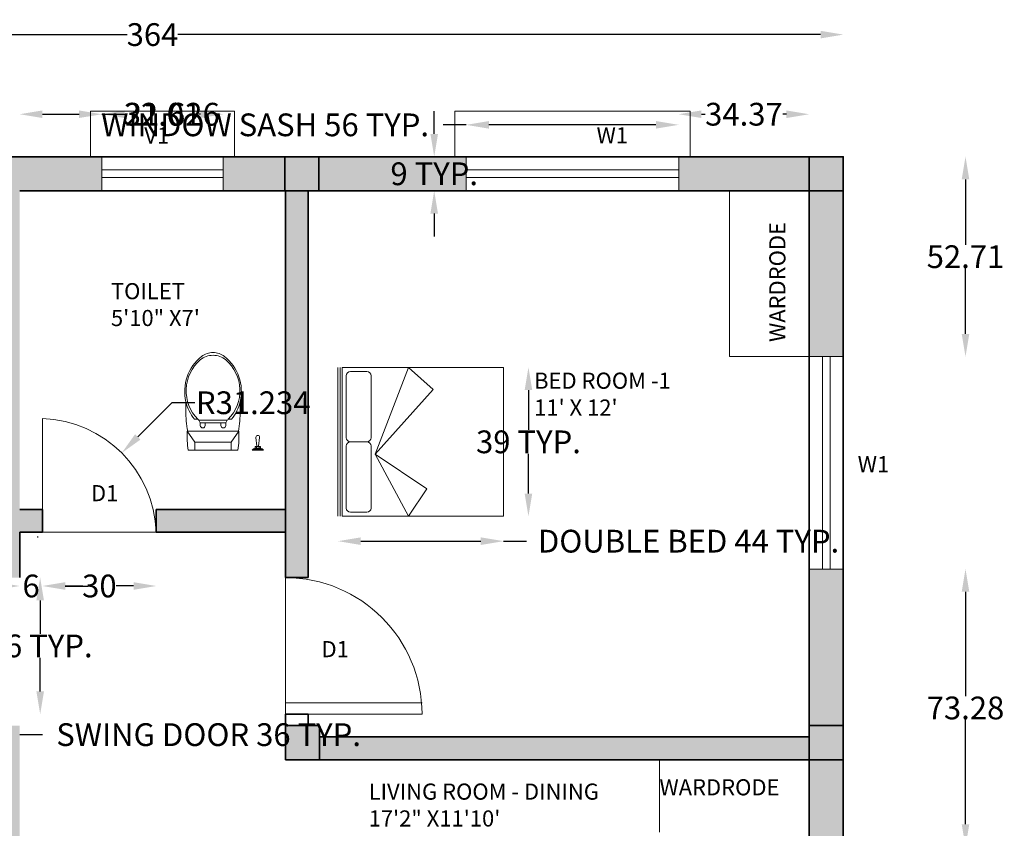
# Model space of a CAD drawing. Units: inches. Extents: x 1994 to 3075, y 3517 to 3950.
# Tile 58 of 58: x 2816 to 3075, y 3737 to 3950. Entities that reach past the tile are written whole.
import ezdxf

# ---------------------------------------------------------------- set-up
doc = ezdxf.new("R2010")
doc.units = ezdxf.units.IN
for name, color, linetype, lineweight in [('A-ANNO-DIMS', 2, 'Continuous', 18), ('A-ANNO-TEXT', 7, 'Continuous', 18), ('A-AREA-IDEN', 7, 'Continuous', 18), ('A-COLS', 7, 'Continuous', 35), ('A-COLS-PATT', 6, 'Continuous', 13), ('A-DOOR', 3, 'Continuous', 18), ('A-FLOR-CASE', 8, 'Continuous', 18), ('A-FURN', 8, 'Continuous', 18), ('A-GLAZ', 4, 'Continuous', 18), ('A-GLAZ-PROJ', 4, 'Continuous', 18), ('A-WALL', 7, 'Continuous', 35), ('A-WALL-PATT', 252, 'Continuous', 13), ('WC-Detail_dwgmodels.com', 8, 'Continuous', 13), ('WC-Outline_dwgmodels.com', 8, 'Continuous', 18)]:
    doc.layers.add(name, color=color, linetype=linetype, lineweight=lineweight)
doc.styles.get("Standard").update_dxf_attribs({"font": 'arial.ttf'})
doc.dimstyles.get("Standard").update_dxf_attribs({"dimtxt": 6, "dimasz": 6, "dimexe": 0.18, "dimexo": 0.0625, "dimgap": 0.09, "dimtad": 0, "dimtih": 1, "dimtoh": 1, "dimdec": 4, "dimzin": 0, "dimdsep": 46, "dimlunit": 4, "dimtxsty": 'Standard', "dimcen": 0.09, "dimse1": 1, "dimse2": 1, "dimadec": 0, "dimazin": 0, "dimtfac": 1, "dimtdec": 4, "dimtofl": 0, "dimtmove": 0, "dimatfit": 3, "dimfxl": 1, "dimtolj": 1, "dimtzin": 0, "dimarcsym": 0})

# ---------------------------------------------------------------- blocks, each defined once
blk = doc.blocks.new('DOOR-SWING-36IN')
for p, q in [((36, 0), (36, 36)), ((36, 36), (36, 0)), ((0, 3), (36, 3)), ((36, 0), (0, 0)), ((0, 0), (36, 0))]:
    blk.add_line(p, q)
blk.add_arc((36, 0), 36, 90, 180)
blk = doc.blocks.new('BED-DOUBLE-PLAN')
for p, q in [((0, 39.28), (0, 0)), ((0.55, 0), (0.55, 39.28)), ((1.09, 0), (1.09, 39.28)), ((1.09, 39.28), (43.64, 39.28)), ((9.82, 16.37), (18.55, 39.28)), ((25.06, 33.47), (18.55, 39.28)), ((43.64, 39.28), (43.64, 0)), ((2.18, 20.73), (2.18, 37.09)), ((3.27, 38.19), (7.64, 38.19)), ((8.73, 20.73), (8.73, 37.09)), ((9.82, 16.37), (25.06, 33.47)), ((2.18, 2.18), (2.18, 18.55)), ((7.64, 19.64), (3.27, 19.64)), ((8.73, 2.18), (8.73, 18.55)), ((18.55, 0), (9.82, 16.37)), ((23.41, 7.25), (9.82, 16.37)), ((18.55, 0), (23.41, 7.25)), ((7.64, 1.09), (3.27, 1.09)), ((43.64, 0), (1.09, 0))]:
    blk.add_line(p, q)
for centre, start, end in [((3.27, 37.09), 90, 180), ((7.64, 37.09), 0, 90), ((3.27, 20.73), 180, 270), ((3.27, 18.55), 90, 180), ((7.64, 20.73), 270, 0), ((7.64, 18.55), 0, 90), ((3.27, 2.18), 180, 270), ((7.64, 2.18), 270, 0)]:
    blk.add_arc(centre, 1.09, start, end)
blk = doc.blocks.new('WINDOW-56IN-SASH')
for p, q in [((56.01, 9), (0, 9)), ((0, 5.5), (56.01, 5.5)), ((0, 3.5), (56.01, 3.5)), ((0, 0), (56.01, 0))]:
    blk.add_line(p, q)
blk = doc.blocks.new('WINDOW-HOOD-62IN')
for p, q in [((0, 59.01), (0, 62.01)), ((0, 62.01), (12, 62.01)), ((0, 0), (0, 59.01)), ((12, 0), (0, 0))]:
    blk.add_line(p, q)
blk = doc.blocks.new('*D17')
at = {"layer": 'A-ANNO-DIMS', "color": 0, "lineweight": -2, "transparency": 16777216}
for p, q in [((2933.69, 3922.53), (2927.69, 3922.53)), ((2983.7, 3922.53), (2939.69, 3922.53))]:
    blk.add_line(p, q, dxfattribs=at)
at = {"layer": 'A-ANNO-DIMS', "color": 0, "transparency": 16777216}
for points in [[(2939.69, 3923.53), (2939.69, 3921.53), (2933.69, 3922.53)], [(2983.7, 3923.53), (2983.7, 3921.53), (2989.7, 3922.53)]]:
    blk.add_solid(points, dxfattribs=at)
at = {"layer": 'Defpoints', "color": 0, "transparency": 16777216}
for p in [(2933.69, 3922.53), (2933.69, 3914.13), (2989.7, 3914.13)]:
    blk.add_point(p, dxfattribs=at)
at = {"layer": 'A-ANNO-DIMS', "color": 0, "transparency": 16777216, "insert": (2880.74, 3922.53), "char_height": 6, "attachment_point": 5}
blk.add_mtext('\\A1;WINDOW SASH 56 TYP.', dxfattribs=at)
blk = doc.blocks.new('*D18')
at = {"layer": 'A-ANNO-DIMS', "color": 0, "lineweight": -2, "transparency": 16777216}
for p, q in [((2925.29, 3920.13), (2925.29, 3926.13)), ((2925.29, 3899.13), (2925.29, 3893.13))]:
    blk.add_line(p, q, dxfattribs=at)
at = {"layer": 'A-ANNO-DIMS', "color": 0, "transparency": 16777216}
for points in [[(2924.29, 3920.13), (2926.29, 3920.13), (2925.29, 3914.13)], [(2924.29, 3899.13), (2926.29, 3899.13), (2925.29, 3905.13)]]:
    blk.add_solid(points, dxfattribs=at)
at = {"layer": 'Defpoints', "color": 0, "transparency": 16777216}
for p in [(2933.69, 3914.13), (2925.29, 3905.13), (2933.69, 3905.13)]:
    blk.add_point(p, dxfattribs=at)
at = {"layer": 'A-ANNO-DIMS', "color": 0, "transparency": 16777216, "insert": (2925.29, 3909.63), "char_height": 6, "attachment_point": 5}
blk.add_mtext('\\A1;9 TYP.', dxfattribs=at)
blk = doc.blocks.new('*D21')
at = {"layer": 'A-ANNO-DIMS', "color": 0, "lineweight": -2, "transparency": 16777216}
for p, q in [((2786.07, 3761.73), (2810.07, 3761.73)), ((2816.07, 3761.73), (2822.07, 3761.73))]:
    blk.add_line(p, q, dxfattribs=at)
at = {"layer": 'A-ANNO-DIMS', "color": 0, "transparency": 16777216}
for points in [[(2786.07, 3762.73), (2786.07, 3760.73), (2780.07, 3761.73)], [(2810.07, 3762.73), (2810.07, 3760.73), (2816.07, 3761.73)]]:
    blk.add_solid(points, dxfattribs=at)
at = {"layer": 'Defpoints', "color": 0, "transparency": 16777216}
for p in [(2780.07, 3767.13), (2816.07, 3767.13), (2816.07, 3761.73)]:
    blk.add_point(p, dxfattribs=at)
at = {"layer": 'A-ANNO-DIMS', "color": 0, "transparency": 16777216, "insert": (2865.85, 3761.73), "char_height": 6, "attachment_point": 5}
blk.add_mtext('\\A1;SWING DOOR 36 TYP.', dxfattribs=at)
blk = doc.blocks.new('*D22')
at = {"layer": 'A-ANNO-DIMS', "color": 0, "lineweight": -2, "transparency": 16777216}
for p, q in [((2821.47, 3797.13), (2821.47, 3788.28)), ((2821.47, 3773.13), (2821.47, 3781.97))]:
    blk.add_line(p, q, dxfattribs=at)
at = {"layer": 'A-ANNO-DIMS', "color": 0, "transparency": 16777216}
for points in [[(2820.47, 3797.13), (2822.47, 3797.13), (2821.47, 3803.13)], [(2820.47, 3773.13), (2822.47, 3773.13), (2821.47, 3767.13)]]:
    blk.add_solid(points, dxfattribs=at)
at = {"layer": 'Defpoints', "color": 0, "transparency": 16777216}
for p in [(2816.07, 3803.13), (2821.47, 3803.13), (2816.07, 3767.13)]:
    blk.add_point(p, dxfattribs=at)
at = {"layer": 'A-ANNO-DIMS', "color": 0, "transparency": 16777216, "insert": (2821.47, 3785.13), "char_height": 6, "attachment_point": 5}
blk.add_mtext('\\A1;36 TYP.', dxfattribs=at)
blk = doc.blocks.new('*D23')
at = {"layer": 'A-ANNO-DIMS', "color": 0, "lineweight": -2, "transparency": 16777216}
for p, q in [((2905.93, 3812.75), (2937.57, 3812.75)), ((2943.57, 3812.75), (2949.57, 3812.75))]:
    blk.add_line(p, q, dxfattribs=at)
at = {"layer": 'A-ANNO-DIMS', "color": 0, "transparency": 16777216}
for points in [[(2905.93, 3813.75), (2905.93, 3811.75), (2899.93, 3812.75)], [(2937.57, 3813.75), (2937.57, 3811.75), (2943.57, 3812.75)]]:
    blk.add_solid(points, dxfattribs=at)
at = {"layer": 'Defpoints', "color": 0, "transparency": 16777216}
for p in [(2899.93, 3819.3), (2943.57, 3819.3), (2943.57, 3812.75)]:
    blk.add_point(p, dxfattribs=at)
at = {"layer": 'A-ANNO-DIMS', "color": 0, "transparency": 16777216, "insert": (2992.3, 3812.75), "char_height": 6, "attachment_point": 5}
blk.add_mtext('\\A1;DOUBLE BED 44 TYP.', dxfattribs=at)
blk = doc.blocks.new('*D24')
at = {"layer": 'A-ANNO-DIMS', "color": 0, "lineweight": -2, "transparency": 16777216}
for p, q in [((2950.12, 3852.58), (2950.12, 3842.09)), ((2950.12, 3825.3), (2950.12, 3835.78))]:
    blk.add_line(p, q, dxfattribs=at)
at = {"layer": 'A-ANNO-DIMS', "color": 0, "transparency": 16777216}
for points in [[(2949.12, 3852.58), (2951.12, 3852.58), (2950.12, 3858.58)], [(2949.12, 3825.3), (2951.12, 3825.3), (2950.12, 3819.3)]]:
    blk.add_solid(points, dxfattribs=at)
at = {"layer": 'Defpoints', "color": 0, "transparency": 16777216}
for p in [(2943.57, 3858.58), (2950.12, 3858.58), (2943.57, 3819.3)]:
    blk.add_point(p, dxfattribs=at)
at = {"layer": 'A-ANNO-DIMS', "color": 0, "transparency": 16777216, "insert": (2950.12, 3838.94), "char_height": 6, "attachment_point": 5}
blk.add_mtext('\\A1;39 TYP.', dxfattribs=at)
blk = doc.blocks.new('*D31')
at = {"layer": 'A-ANNO-DIMS', "color": 0, "lineweight": -2, "transparency": 16777216}
for p, q in [((2675.07, 3946.33), (2844.37, 3946.33)), ((3027.07, 3946.33), (2857.78, 3946.33))]:
    blk.add_line(p, q, dxfattribs=at)
at = {"layer": 'A-ANNO-DIMS', "color": 0, "transparency": 16777216}
for points in [[(2675.07, 3947.33), (2675.07, 3945.33), (2669.07, 3946.33)], [(3027.07, 3947.33), (3027.07, 3945.33), (3033.07, 3946.33)]]:
    blk.add_solid(points, dxfattribs=at)
at = {"layer": 'Defpoints', "color": 0, "transparency": 16777216}
for p in [(3033.07, 3946.33), (2669.07, 3914.13), (3033.07, 3914.13)]:
    blk.add_point(p, dxfattribs=at)
at = {"layer": 'A-ANNO-DIMS', "color": 0, "transparency": 16777216, "insert": (2851.07, 3946.33), "char_height": 6, "attachment_point": 5}
blk.add_mtext('\\A1;364', dxfattribs=at)
blk = doc.blocks.new('*D38')
at = {"layer": 'A-ANNO-DIMS', "color": 0, "lineweight": -2, "transparency": 16777216}
for p, q in [((3065.27, 3799.41), (3065.27, 3771.92)), ((3065.27, 3738.12), (3065.27, 3765.61))]:
    blk.add_line(p, q, dxfattribs=at)
at = {"layer": 'A-ANNO-DIMS', "color": 0, "transparency": 16777216}
for points in [[(3064.27, 3799.41), (3066.27, 3799.41), (3065.27, 3805.41)], [(3064.27, 3738.12), (3066.27, 3738.12), (3065.27, 3732.12)]]:
    blk.add_solid(points, dxfattribs=at)
at = {"layer": 'Defpoints', "color": 0, "transparency": 16777216}
for p in [(3033.07, 3805.41), (3065.27, 3805.41), (3033.07, 3732.12)]:
    blk.add_point(p, dxfattribs=at)
at = {"layer": 'A-ANNO-DIMS', "color": 0, "transparency": 16777216, "insert": (3065.27, 3768.77), "char_height": 6, "attachment_point": 5}
blk.add_mtext('\\A1;73.28', dxfattribs=at)
blk = doc.blocks.new('*D39')
at = {"layer": 'A-ANNO-DIMS', "color": 0, "lineweight": -2, "transparency": 16777216}
for p, q in [((3065.27, 3908.13), (3065.27, 3890.93)), ((3065.27, 3867.42), (3065.27, 3884.62))]:
    blk.add_line(p, q, dxfattribs=at)
at = {"layer": 'A-ANNO-DIMS', "color": 0, "transparency": 16777216}
for points in [[(3064.27, 3908.13), (3066.27, 3908.13), (3065.27, 3914.13)], [(3064.27, 3867.42), (3066.27, 3867.42), (3065.27, 3861.42)]]:
    blk.add_solid(points, dxfattribs=at)
at = {"layer": 'Defpoints', "color": 0, "transparency": 16777216}
for p in [(3033.07, 3914.13), (3065.27, 3914.13), (3033.07, 3861.42)]:
    blk.add_point(p, dxfattribs=at)
at = {"layer": 'A-ANNO-DIMS', "color": 0, "transparency": 16777216, "insert": (3065.27, 3887.77), "char_height": 6, "attachment_point": 5}
blk.add_mtext('\\A1;52.71', dxfattribs=at)
blk = doc.blocks.new('*D41')
at = {"layer": 'A-ANNO-DIMS', "color": 0, "lineweight": -2, "transparency": 16777216}
for p, q in [((2822.07, 3925.33), (2831.7, 3925.33)), ((2837.7, 3925.33), (2843.7, 3925.33))]:
    blk.add_line(p, q, dxfattribs=at)
at = {"layer": 'A-ANNO-DIMS', "color": 0, "transparency": 16777216}
for points in [[(2822.07, 3926.33), (2822.07, 3924.33), (2816.07, 3925.33)], [(2831.7, 3926.33), (2831.7, 3924.33), (2837.7, 3925.33)]]:
    blk.add_solid(points, dxfattribs=at)
at = {"layer": 'Defpoints', "color": 0, "transparency": 16777216}
for p in [(2837.7, 3925.33), (2816.07, 3905.13), (2837.7, 3905.13)]:
    blk.add_point(p, dxfattribs=at)
at = {"layer": 'A-ANNO-DIMS', "color": 0, "transparency": 16777216, "insert": (2856.29, 3925.33), "char_height": 6, "attachment_point": 5}
blk.add_mtext('\\A1;21.626', dxfattribs=at)
blk = doc.blocks.new('*D42')
at = {"layer": 'A-ANNO-DIMS', "color": 0, "lineweight": -2, "transparency": 16777216}
for p, q in [((2843.7, 3925.33), (2844.07, 3925.33)), ((2863.71, 3925.33), (2863.34, 3925.33))]:
    blk.add_line(p, q, dxfattribs=at)
at = {"layer": 'A-ANNO-DIMS', "color": 0, "transparency": 16777216}
for points in [[(2843.7, 3926.33), (2843.7, 3924.33), (2837.7, 3925.33)], [(2863.71, 3926.33), (2863.71, 3924.33), (2869.71, 3925.33)]]:
    blk.add_solid(points, dxfattribs=at)
at = {"layer": 'Defpoints', "color": 0, "transparency": 16777216}
for p in [(2869.71, 3925.33), (2837.7, 3905.13), (2869.71, 3905.13)]:
    blk.add_point(p, dxfattribs=at)
at = {"layer": 'A-ANNO-DIMS', "color": 0, "transparency": 16777216, "insert": (2853.7, 3925.33), "char_height": 6, "attachment_point": 5}
blk.add_mtext('\\A1;32.01', dxfattribs=at)
blk = doc.blocks.new('*D43')
at = {"layer": 'A-ANNO-DIMS', "color": 0, "lineweight": -2, "transparency": 16777216}
for p, q in [((2995.7, 3925.33), (2996.68, 3925.33)), ((3018.07, 3925.33), (3017.1, 3925.33))]:
    blk.add_line(p, q, dxfattribs=at)
at = {"layer": 'A-ANNO-DIMS', "color": 0, "transparency": 16777216}
for points in [[(2995.7, 3926.33), (2995.7, 3924.33), (2989.7, 3925.33)], [(3018.07, 3926.33), (3018.07, 3924.33), (3024.07, 3925.33)]]:
    blk.add_solid(points, dxfattribs=at)
at = {"layer": 'Defpoints', "color": 0, "transparency": 16777216}
for p in [(3024.07, 3925.33), (2989.7, 3905.13), (3024.07, 3905.13)]:
    blk.add_point(p, dxfattribs=at)
at = {"layer": 'A-ANNO-DIMS', "color": 0, "transparency": 16777216, "insert": (3006.89, 3925.33), "char_height": 6, "attachment_point": 5}
blk.add_mtext('\\A1;34.37', dxfattribs=at)
blk = doc.blocks.new('*D50')
at = {"layer": 'A-ANNO-DIMS', "color": 0, "lineweight": -2, "transparency": 16777216}
for p, q in [((2828.07, 3800.93), (2832.7, 3800.93)), ((2846.07, 3800.93), (2841.45, 3800.93))]:
    blk.add_line(p, q, dxfattribs=at)
at = {"layer": 'A-ANNO-DIMS', "color": 0, "transparency": 16777216}
for points in [[(2828.07, 3801.93), (2828.07, 3799.93), (2822.07, 3800.93)], [(2846.07, 3801.93), (2846.07, 3799.93), (2852.07, 3800.93)]]:
    blk.add_solid(points, dxfattribs=at)
at = {"layer": 'Defpoints', "color": 0, "transparency": 16777216}
for p in [(2822.07, 3821.13), (2852.07, 3821.13), (2822.07, 3800.93)]:
    blk.add_point(p, dxfattribs=at)
at = {"layer": 'A-ANNO-DIMS', "color": 0, "transparency": 16777216, "insert": (2837.07, 3800.93), "char_height": 6, "attachment_point": 5}
blk.add_mtext('\\A1;30', dxfattribs=at)
blk = doc.blocks.new('*D51')
at = {"layer": 'A-ANNO-DIMS', "color": 0, "lineweight": -2, "transparency": 16777216}
for p, q in [((2810.072038, 3800.926884), (2804.072038, 3800.926884)), ((2828.072038, 3800.926884), (2834.072038, 3800.926884))]:
    blk.add_line(p, q, dxfattribs=at)
at = {"layer": 'A-ANNO-DIMS', "color": 0, "transparency": 16777216}
for points in [[(2810.072038, 3801.926884), (2810.072038, 3799.926884), (2816.072038, 3800.926884)], [(2828.072038, 3801.926884), (2828.072038, 3799.926884), (2822.072038, 3800.926884)]]:
    blk.add_solid(points, dxfattribs=at)
at = {"layer": 'Defpoints', "color": 0, "transparency": 16777216}
for p in [(2816.072038, 3821.126884), (2822.072038, 3821.126884), (2816.072038, 3800.926884)]:
    blk.add_point(p, dxfattribs=at)
at = {"layer": 'A-ANNO-DIMS', "color": 0, "transparency": 16777216, "insert": (2819.072038, 3800.926884), "char_height": 6, "attachment_point": 5}
blk.add_mtext('\\A1;6', dxfattribs=at)
blk = doc.blocks.new('*D55')
at = {"layer": 'A-ANNO-DIMS', "color": 0, "lineweight": -2, "transparency": 16777216}
for p, q in [((2856.2, 3849.25), (2847.19, 3840.24)), ((2862.2, 3849.25), (2856.2, 3849.25)), ((2820.77, 3813.92), (2820.95, 3813.92)), ((2820.86, 3813.83), (2820.86, 3814.01))]:
    blk.add_line(p, q, dxfattribs=at)
at = {"layer": 'A-ANNO-DIMS', "color": 0, "transparency": 16777216}
blk.add_solid([(2846.48, 3840.95), (2847.9, 3839.54), (2842.95, 3836)], dxfattribs=at)
at = {"layer": 'Defpoints', "color": 0, "transparency": 16777216}
for p in [(2842.95, 3836), (2820.86, 3813.92)]:
    blk.add_point(p, dxfattribs=at)
at = {"layer": 'A-ANNO-DIMS', "color": 0, "transparency": 16777216, "insert": (2877.6, 3849.25), "char_height": 6, "attachment_point": 5}
blk.add_mtext('\\A1;R31.234', dxfattribs=at)

msp = doc.modelspace()

# ---------------------------------------------------------------- hatches: boundary and pattern name
at = {"layer": 'A-COLS-PATT'}
h = msp.add_hatch(color=256, dxfattribs=at)
h.dxf.hatch_style = 1
h.paths.add_polyline_path([(2678.072, 3914.1269), (2669.072, 3914.1269), (2669.072, 3905.1269), (2678.072, 3905.1269)])
h.paths.add_polyline_path([(2816.072, 3914.1269), (2807.072, 3914.1269), (2807.072, 3905.1269), (2816.072, 3905.1269)])
h.paths.add_polyline_path([(2894.9096, 3914.1269), (2885.9096, 3914.1269), (2885.9096, 3905.1269), (2894.9096, 3905.1269)])
h.paths.add_polyline_path([(3033.072, 3914.1269), (3024.072, 3914.1269), (3024.072, 3905.1269), (3033.072, 3905.1269)])
h.paths.add_polyline_path([(3033.072, 3764.1269), (3024.072, 3764.1269), (3024.072, 3755.1269), (3033.072, 3755.1269)])
h.paths.add_polyline_path([(2895.072, 3764.1269), (2886.072, 3764.1269), (2886.072, 3755.1269), (2895.072, 3755.1269)])
h.paths.add_polyline_path([(2816.072, 3764.1269), (2807.072, 3764.1269), (2807.072, 3755.1269), (2816.072, 3755.1269)])
h.paths.add_polyline_path([(2678.072, 3764.1269), (2669.072, 3764.1269), (2669.072, 3755.1269), (2678.072, 3755.1269)])
h.paths.add_polyline_path([(2678.072, 3664.1269), (2669.072, 3664.1269), (2669.072, 3655.1269), (2678.072, 3655.1269)])
h.paths.add_polyline_path([(2816.072, 3664.1269), (2807.072, 3664.1269), (2807.072, 3655.1269), (2816.072, 3655.1269)])
h.paths.add_polyline_path([(3033.072, 3616.1269), (3024.072, 3616.1269), (3024.072, 3607.1269), (3033.072, 3607.1269)])
h.paths.add_polyline_path([(2894.9096, 3616.1269), (2885.9096, 3616.1269), (2885.9096, 3607.1269), (2894.9096, 3607.1269)])
h.paths.add_polyline_path([(2816.072, 3559.1269), (2807.072, 3559.1269), (2807.072, 3550.1269), (2816.072, 3550.1269)])
h.paths.add_polyline_path([(2678.072, 3559.1269), (2669.072, 3559.1269), (2669.072, 3550.1269), (2678.072, 3550.1269)])
at = {"layer": 'A-WALL-PATT'}
h = msp.add_hatch(color=256, dxfattribs=at)
h.dxf.hatch_style = 1
h.paths.add_polyline_path([(2678.072, 3755.1269), (2669.072, 3755.1269), (2669.072, 3718.5523), (2678.072, 3718.5523)])
h.paths.add_polyline_path([(2807.072, 3761.1269), (2678.072, 3761.1269), (2678.072, 3755.1269), (2807.072, 3755.1269)])
h.paths.add_polyline_path([(2678.072, 3812.7371), (2669.072, 3812.7371), (2669.072, 3809.7371), (2669.072, 3764.1269), (2678.072, 3764.1269)])
h.paths.add_polyline_path([(2678.072, 3905.1269), (2669.072, 3905.1269), (2669.072, 3868.7491), (2678.072, 3868.7491)])
h.paths.add_polyline_path([(2723.826, 3914.1269), (2720.826, 3914.1269), (2678.072, 3914.1269), (2678.072, 3905.1269), (2723.826, 3905.1269)])
h.paths.add_polyline_path([(2807.072, 3914.1269), (2779.838, 3914.1269), (2779.838, 3905.1269), (2807.072, 3905.1269)])
h.paths.add_polyline_path([(2837.6979, 3914.1269), (2834.6979, 3914.1269), (2820.9062, 3914.1269), (2816.072, 3914.1269), (2816.072, 3905.1269), (2837.6979, 3905.1269)])
h.paths.add_polyline_path([(2885.9096, 3914.1269), (2869.71, 3914.1269), (2869.71, 3905.1269), (2876.9183, 3905.1269), (2885.9096, 3905.1269)])
h.paths.add_polyline_path([(2933.6904, 3914.1269), (2930.6904, 3914.1269), (2894.9096, 3914.1269), (2894.9096, 3905.1269), (2933.6904, 3905.1269)])
h.paths.add_polyline_path([(3024.072, 3914.1269), (2989.7025, 3914.1269), (2989.7025, 3905.1269), (3024.072, 3905.1269)])
h.paths.add_polyline_path([(3033.072, 3905.1269), (3024.072, 3905.1269), (3024.072, 3861.4192), (3033.072, 3861.4192)])
h.paths.add_polyline_path([(3033.072, 3805.4072), (3024.072, 3805.4072), (3024.072, 3764.1269), (3033.072, 3764.1269)])
h.paths.add_polyline_path([(3033.072, 3755.1269), (3024.072, 3755.1269), (3024.072, 3732.1247), (3033.072, 3732.1247), (3033.072, 3735.1247)])
h.paths.add_polyline_path([(3024.072, 3761.1269), (2895.072, 3761.1269), (2895.072, 3755.1269), (3024.072, 3755.1269)])
h.paths.add_polyline_path([(3033.072, 3676.1126), (3024.072, 3676.1126), (3024.072, 3616.1269), (3033.072, 3616.1269)])
h.paths.add_polyline_path([(3024.072, 3613.1269), (2959.4908, 3613.1269), (2959.4908, 3607.1269), (3024.072, 3607.1269)])
h.paths.add_polyline_path([(2914.1254, 3613.1269), (2894.9096, 3613.1269), (2894.9096, 3607.1269), (2914.1254, 3607.1269)])
h.paths.add_polyline_path([(2885.9096, 3613.1269), (2852.072, 3613.1269), (2852.072, 3607.1269), (2885.9096, 3607.1269)])
h.paths.add_polyline_path([(2822.072, 3613.1269), (2810.072, 3613.1269), (2810.072, 3559.1269), (2816.072, 3559.1269), (2816.072, 3607.1269), (2822.072, 3607.1269)])
h.paths.add_polyline_path([(2933.072, 3607.1269), (2924.072, 3607.1269), (2924.072, 3550.1269), (2892.072, 3550.1269), (2816.072, 3550.1269), (2810.072, 3550.1269), (2810.072, 3541.1269), (2892.072, 3541.1269), (2933.072, 3541.1269)])
h.paths.add_polyline_path([(2807.072, 3559.1269), (2678.072, 3559.1269), (2678.072, 3550.1269), (2807.072, 3550.1269)])
h.paths.add_polyline_path([(2678.072, 3655.1269), (2669.072, 3655.1269), (2669.072, 3559.1269), (2678.072, 3559.1269)])
h.paths.add_polyline_path([(2678.072, 3686.5403), (2669.072, 3686.5403), (2669.072, 3664.1269), (2678.072, 3664.1269)])
h.paths.add_polyline_path([(2807.072, 3661.1269), (2678.072, 3661.1269), (2678.072, 3655.1269), (2807.072, 3655.1269)])
h.paths.add_polyline_path([(2816.072, 3755.1269), (2810.072, 3755.1269), (2810.072, 3703.1269), (2816.072, 3703.1269)])
h.paths.add_polyline_path([(2816.072, 3905.1269), (2810.072, 3905.1269), (2810.072, 3803.1269), (2816.072, 3803.1269), (2816.072, 3815.1269)])
h.paths.add_polyline_path([(2886.072, 3821.1269), (2852.072, 3821.1269), (2852.072, 3815.1269), (2886.072, 3815.1269)])
h.paths.add_polyline_path([(2822.072, 3821.1269), (2816.072, 3821.1269), (2816.072, 3815.1269), (2822.072, 3815.1269)])
h.paths.add_polyline_path([(2892.072, 3905.1269), (2886.072, 3905.1269), (2886.072, 3803.1269), (2892.072, 3803.1269)])

# ---------------------------------------------------------------- linework, layer by layer
at = {"layer": 'A-COLS'}
for points in [[(2885.9096, 3905.1269), (2894.9096, 3905.1269), (2894.9096, 3914.1269), (2885.9096, 3914.1269)], [(3024.072, 3905.1269), (3033.072, 3905.1269), (3033.072, 3914.1269), (3024.072, 3914.1269)], [(2886.072, 3755.1269), (2895.072, 3755.1269), (2895.072, 3764.1269), (2886.072, 3764.1269)], [(3024.072, 3755.1269), (3033.072, 3755.1269), (3033.072, 3764.1269), (3024.072, 3764.1269)]]:
    msp.add_lwpolyline(points, close=True, dxfattribs=at)
at = {"layer": 'A-DOOR'}
for q in [(2822.072, 3845.1269), (2852.072, 3815.1269)]:
    msp.add_line((2822.072, 3815.1269), q, dxfattribs=at)
msp.add_arc((2820.861, 3813.9159), 31.2345, 2.22198, 87.77802, dxfattribs=at)
at = {"layer": 'A-FLOR-CASE'}
for p, q in [((3024.072, 3905.1269), (3003.097, 3905.1269)), ((3003.097, 3905.1269), (3003.097, 3861.4192)), ((3003.097, 3861.4192), (3024.072, 3861.4192)), ((2984.6205, 3755.1269), (2984.6205, 3736.0298))]:
    msp.add_line(p, q, dxfattribs=at)
at = {"layer": 'A-GLAZ'}
for p, q in [((2876.9183, 3914.1269), (2820.9062, 3914.1269)), ((2837.6979, 3914.1269), (2837.6979, 3905.1269)), ((2869.71, 3905.1269), (2869.71, 3914.1269)), ((2933.6904, 3914.1269), (2933.6904, 3905.1269)), ((2989.7025, 3905.1269), (2989.7025, 3914.1269)), ((2837.6979, 3910.6269), (2869.71, 3910.6269)), ((2837.6979, 3908.6269), (2869.71, 3908.6269)), ((2820.9062, 3905.1269), (2876.9183, 3905.1269)), ((3033.072, 3861.4192), (3024.072, 3861.4192)), ((3024.072, 3805.4072), (3033.072, 3805.4072))]:
    msp.add_line(p, q, dxfattribs=at)
at = {"layer": 'A-GLAZ-PROJ'}
for p, q in [((2834.6979, 3914.1269), (2834.6979, 3926.1269)), ((2834.6979, 3926.1269), (2869.71, 3926.1269)), ((2869.71, 3926.1269), (2872.71, 3926.1269)), ((2872.71, 3926.1269), (2872.71, 3914.1269)), ((2837.6979, 3914.1269), (2834.6979, 3914.1269)), ((2933.6904, 3914.1269), (2930.6904, 3914.1269))]:
    msp.add_line(p, q, dxfattribs=at)
at = {"layer": 'A-WALL'}
for p, q in [((2669.072, 3914.1269), (3033.072, 3914.1269)), ((3033.072, 3914.1269), (3033.072, 3607.1269)), ((2816.072, 3905.1269), (2886.072, 3905.1269)), ((2886.072, 3905.1269), (2886.072, 3803.1269)), ((2892.072, 3905.1269), (2892.072, 3803.1269)), ((2892.072, 3905.1269), (3024.072, 3905.1269)), ((3024.072, 3905.1269), (3024.072, 3607.1269)), ((2816.072, 3821.1269), (2822.072, 3821.1269)), ((2816.072, 3821.1269), (2822.072, 3821.1269)), ((2822.072, 3821.1269), (2822.072, 3815.1269)), ((2852.072, 3815.1269), (2852.072, 3821.1269)), ((2852.072, 3821.1269), (2886.072, 3821.1269)), ((2816.072, 3815.1269), (2822.072, 3815.1269)), ((2816.072, 3815.1269), (2816.072, 3803.1269)), ((2852.072, 3815.1269), (2886.072, 3815.1269)), ((2886.072, 3803.1269), (2892.072, 3803.1269)), ((2886.072, 3803.1269), (2892.072, 3803.1269)), ((2892.072, 3767.1269), (2886.072, 3767.1269)), ((2886.072, 3767.1269), (2886.072, 3755.1269)), ((2892.072, 3767.1269), (2886.072, 3767.1269)), ((2892.072, 3764.1269), (2892.072, 3767.1269)), ((2892.072, 3767.1269), (2892.072, 3764.1269)), ((2895.072, 3761.1269), (3024.072, 3761.1269)), ((2892.2345, 3755.1269), (2886.2345, 3755.1269)), ((2892.072, 3755.1269), (3024.072, 3755.1269))]:
    msp.add_line(p, q, dxfattribs=at)
at = {"layer": 'WC-Detail_dwgmodels.com'}
for p, q in [((2863.2942, 3844.6393), (2863.6539, 3843.9789)), ((2864.9442, 3843.9789), (2863.6539, 3843.9789)), ((2863.6539, 3843.9789), (2863.6539, 3843.2584)), ((2864.9442, 3843.2584), (2864.9442, 3843.9789)), ((2867.0129, 3843.9789), (2864.9442, 3843.9789)), ((2867.0129, 3843.9789), (2869.0817, 3843.9789)), ((2869.0817, 3843.2584), (2869.0817, 3843.9789)), ((2869.0817, 3843.9789), (2870.372, 3843.9789)), ((2870.7317, 3844.6393), (2870.372, 3843.9789)), ((2870.372, 3843.9789), (2870.372, 3843.2584))]:
    msp.add_line(p, q, dxfattribs=at)
for points in [[(2863.019, 3844.9083, -0.43421705), (2863.6539, 3860.544, -0.18263377), (2867.0129, 3861.7687, -2.69381511)], [(2871.0069, 3844.9083, 0.43421705), (2870.372, 3860.544, 0.18263377), (2867.0129, 3861.7687, 2.69381511)], [(2862.1239, 3844.9083, -0.11024028), (2859.8696, 3849.5008, -0.16845003)], [(2871.902, 3844.9083, 0.11024028), (2874.1563, 3849.5008, 0.16845003)], [(2863.019, 3844.9083), (2862.1239, 3844.9083, -0.4166064)], [(2863.2942, 3844.6393, -0.00898513), (2863.019, 3844.9083, -0.18263377)], [(2870.7317, 3844.6393, 0.00898513), (2871.0069, 3844.9083, 0.18263377)], [(2871.0069, 3844.9083), (2871.902, 3844.9083, 0.4166064)], [(2867.0129, 3844.6393), (2863.2942, 3844.6393, -0.44493811)], [(2867.0129, 3844.6393), (2870.7317, 3844.6393, 0.00898513)]]:
    msp.add_lwpolyline(points, format="xyb", dxfattribs=at)
for points in [[(2877.5228, 3836.9666), (2880.1161, 3836.9666)], [(2878.1383, 3837.313), (2879.5005, 3837.313)], [(2878.4612, 3837.313), (2878.4612, 3837.7461)], [(2879.1541, 3837.313), (2879.1541, 3837.7461)]]:
    msp.add_lwpolyline(points, dxfattribs=at)
for centre in [(2864.2991, 3843.2584), (2869.7268, 3843.2584)]:
    msp.add_arc(centre, 0.6451, 180, 0, dxfattribs=at)
at = {"layer": 'WC-Outline_dwgmodels.com'}
for points in [[(2859.8696, 3849.5008, -0.29291354), (2864.0137, 3861.4752, -0.16845003), (2867.0129, 3862.5158, -2.88308192)], [(2874.1563, 3849.5008, 0.29291354), (2870.0122, 3861.4752, 0.16845003), (2867.0129, 3862.5158, 2.88308192)], [(2860.3378, 3841.7316, -0.05212142), (2859.8696, 3847.1332), (2859.8696, 3849.5008, -0.14456028)], [(2873.6881, 3841.7316, 0.05212142), (2874.1563, 3847.1332), (2874.1563, 3849.5008, 0.14456028)], [(2860.4882, 3836.7631, -0.05671124), (2860.2118, 3841.7237), (2860.3378, 3841.7237)], [(2873.5377, 3836.7631, 0.05671124), (2873.8141, 3841.7237), (2873.6881, 3841.7237)], [(2878.5911, 3837.7697), (2878.3313, 3840.124, -0.48260727), (2878.8313, 3840.6201, 0.54790474)], [(2879.0242, 3837.7697), (2879.284, 3840.124, 0.48260727), (2878.784, 3840.6201, -0.54790474)], [(2878.1383, 3837.313, 0.15838106), (2877.3391, 3836.767, -2.93238314)], [(2879.5005, 3837.313, -0.15838106), (2880.2998, 3836.767, 2.93238314)]]:
    msp.add_lwpolyline(points, format="xyb", dxfattribs=at)
for points in [[(2860.2118, 3841.7237), (2862.2393, 3838.8891), (2862.2393, 3836.7631)], [(2860.3378, 3841.7237), (2867.0129, 3841.7237)], [(2873.6881, 3841.7237), (2867.0129, 3841.7237)], [(2873.8141, 3841.7237), (2871.7866, 3838.8891), (2871.7866, 3836.7631)], [(2862.2393, 3838.8891), (2867.0129, 3838.8891)], [(2871.7866, 3838.8891), (2867.0129, 3838.8891)], [(2878.5911, 3837.7461), (2878.158, 3837.7461), (2878.1383, 3837.313)], [(2879.0242, 3837.7461), (2878.5911, 3837.7461)], [(2879.5005, 3837.313), (2879.5005, 3837.7461), (2879.0242, 3837.7461)], [(2860.4882, 3836.7631), (2873.5377, 3836.7631)], [(2877.3391, 3836.767), (2880.2998, 3836.767)]]:
    msp.add_lwpolyline(points, dxfattribs=at)

# ---------------------------------------------------------------- block references
at = {"layer": 'A-DOOR', "extrusion": (0, 0, -1), "zscale": -1}
msp.add_blockref('DOOR-SWING-36IN', (-2922.0721, 3767.127), dxfattribs=at)
at = {"layer": 'A-FURN'}
msp.add_blockref('BED-DOUBLE-PLAN', (2899.932, 3819.3), dxfattribs=at)
at = {"layer": 'A-GLAZ'}
for p, rotation in [((2989.7024, 3914.1268), 180), ((3033.0719, 3805.4072), 89.9999999999985)]:
    msp.add_blockref('WINDOW-56IN-SASH', p, dxfattribs=dict(at, rotation=rotation))
at = {"layer": 'A-GLAZ-PROJ', "rotation": 269.9999999999987}
msp.add_blockref('WINDOW-HOOD-62IN', (2930.6903, 3926.1269), dxfattribs=at)

# ---------------------------------------------------------------- texts
at = {"layer": 'A-ANNO-TEXT', "char_height": 4.24528, "attachment_point": 1}
for s, insert in [('V1', (2848.9122, 3921.8555)), ('W1', (2968.0618, 3921.8974)), ('W1', (3036.8705, 3835.1652)), ('D1', (2834.8588, 3827.5334)), ('D1', (2895.5958, 3786.4005)), ('WARDRODE', (2984.6205, 3749.9713))]:
    msp.add_mtext_dynamic_manual_height_columns(s, width=102.693633, gutter_width=21.2264, heights=[0], dxfattribs=dict(at, insert=insert))
at = {"layer": 'A-ANNO-TEXT', "insert": (3013.5845, 3865.259), "char_height": 4.24528, "attachment_point": 1, "rotation": 90}
msp.add_mtext_dynamic_manual_height_columns('WARDRODE', width=102.693633, gutter_width=21.2264, heights=[0], dxfattribs=at)
at = {"layer": 'A-AREA-IDEN', "attachment_point": 1}
for s, width, heights, insert, char_height in [('TOILET\\P5\'10" X7\'', 102.693633, [0], (2840.1157, 3880.7961), 4.24528), ("BED ROOM -1\\P11' X 12'", 112.760675, [22.775], (2951.6129, 3857.1914), 4.245283), ('LIVING ROOM - DINING\\P17\'2" X11\'10\'', 102.693633, [0], (2908.0196, 3748.8317), 4.245283)]:
    msp.add_mtext_dynamic_manual_height_columns(s, width=width, gutter_width=21.2264, heights=heights, dxfattribs=dict(at, insert=insert, char_height=char_height))

# ---------------------------------------------------------------- dimensions: what is measured, and where the dimension line sits
at = {"layer": 'A-ANNO-DIMS'}
for base, p1, p2, override, picture, middle in [((3033.072, 3946.3269), (2669.072, 3914.1269), (3033.072, 3914.1269), {"dimdec": 0, "dimlfac": 1, "dimrnd": 0, "dimzin": 0, "dimdsep": 46, "dimlunit": 2}, '*D31', (2851.072, 3946.3269)), ((2837.6979, 3925.3269), (2816.072, 3905.1269), (2837.6979, 3905.1269), {"dimdec": 3, "dimlfac": 1, "dimrnd": 0, "dimzin": 0, "dimdsep": 46, "dimlunit": 2}, '*D41', (2856.2913, 3925.3269)), ((2869.71, 3925.3269), (2837.6979, 3905.1269), (2869.71, 3905.1269), {"dimdec": 2, "dimlfac": 1, "dimrnd": 0, "dimzin": 0, "dimdsep": 46, "dimlunit": 2}, '*D42', (2853.7039, 3925.3269)), ((3024.072, 3925.3269), (2989.7025, 3905.1269), (3024.072, 3905.1269), {"dimdec": 2, "dimlfac": 1, "dimrnd": 0, "dimzin": 0, "dimdsep": 46, "dimlunit": 2}, '*D43', (3006.8873, 3925.3269))]:
    dim = msp.add_linear_dim(base=base, p1=p1, p2=p2, dimstyle='Standard', override=override, dxfattribs=at)
    dim.commit()
    dim.dimension.update_dxf_attribs({"geometry": picture, "text_midpoint": middle})
for base, p1, p2, angle, text, picture, middle in [((2933.6904, 3922.5287), (2989.7025, 3914.1269), (2933.6904, 3914.1269), 180, 'WINDOW SASH <> TYP.', '*D17', (2880.7443, 3922.5287)), ((2925.2886, 3905.1269), (2933.6904, 3914.1269), (2933.6904, 3905.1269), 270, '<> TYP.', '*D18', (2925.2886, 3909.6269)), ((2950.1195, 3858.5767), (2943.5733, 3819.2996), (2943.5733, 3858.5767), 90, '<> TYP.', '*D24', (2950.1195, 3838.9381)), ((2821.472, 3803.1269), (2816.072, 3767.1269), (2816.072, 3803.1269), 90, '<> TYP.', '*D22', (2821.472, 3785.1269))]:
    dim = msp.add_linear_dim(base=base, p1=p1, p2=p2, angle=angle, text=text, dimstyle='Standard', override={"dimdec": 0, "dimlfac": 1, "dimrnd": 0, "dimzin": 0, "dimdsep": 46, "dimlunit": 2}, dxfattribs=at)
    dim.commit()
    dim.dimension.update_dxf_attribs({"geometry": picture, "text_midpoint": middle})
for base, p1, p2, angle, override, picture, middle in [((3065.272, 3914.1269), (3033.072, 3861.4192), (3033.072, 3914.1269), 90, {"dimdec": 2, "dimlfac": 1, "dimrnd": 0, "dimzin": 0, "dimdsep": 46, "dimlunit": 2}, '*D39', (3065.272, 3887.7731)), ((2816.072, 3800.9269), (2822.072, 3821.1269), (2816.072, 3821.1269), 180, {"dimdec": 0, "dimlfac": 1, "dimrnd": 0, "dimzin": 0, "dimdsep": 46, "dimlunit": 2}, '*D51', (2819.072, 3800.9269)), ((2822.072, 3800.9269), (2852.072, 3821.1269), (2822.072, 3821.1269), 180, {"dimdec": 0, "dimlfac": 1, "dimrnd": 0, "dimzin": 0, "dimdsep": 46, "dimlunit": 2}, '*D50', (2837.072, 3800.9269)), ((3065.272, 3805.4072), (3033.072, 3732.1247), (3033.072, 3805.4072), 90, {"dimdec": 2, "dimlfac": 1, "dimrnd": 0, "dimzin": 0, "dimdsep": 46, "dimlunit": 2}, '*D38', (3065.272, 3768.7659))]:
    dim = msp.add_linear_dim(base=base, p1=p1, p2=p2, angle=angle, dimstyle='Standard', override=override, dxfattribs=at)
    dim.commit()
    dim.dimension.update_dxf_attribs({"geometry": picture, "text_midpoint": middle})
dim = msp.add_radius_dim(center=(2820.86104, 3813.91589), mpoint=(2842.94708, 3836.00208), dimstyle='Standard', override={"dimdec": 3, "dimlfac": 1, "dimrnd": 0, "dimzin": 0, "dimdsep": 46, "dimlunit": 2}, dxfattribs=at)
dim.commit()
dim.dimension.update_dxf_attribs({"geometry": '*D55', "text_midpoint": (2877.6018, 3849.25379), "dimtype": 164})
for base, p1, p2, text, picture, middle in [((2943.5733, 3812.7534), (2899.9321, 3819.2996), (2943.5733, 3819.2996), 'DOUBLE BED <> TYP.', '*D23', (2992.2977, 3812.7534)), ((2816.072, 3761.7269), (2780.072, 3767.1269), (2816.072, 3767.1269), 'SWING DOOR <> TYP.', '*D21', (2865.8544, 3761.7269))]:
    dim = msp.add_linear_dim(base=base, p1=p1, p2=p2, text=text, dimstyle='Standard', override={"dimdec": 0, "dimlfac": 1, "dimrnd": 0, "dimzin": 0, "dimdsep": 46, "dimlunit": 2}, dxfattribs=at)
    dim.commit()
    dim.dimension.update_dxf_attribs({"geometry": picture, "text_midpoint": middle})

doc.saveas('drawing.dxf')
